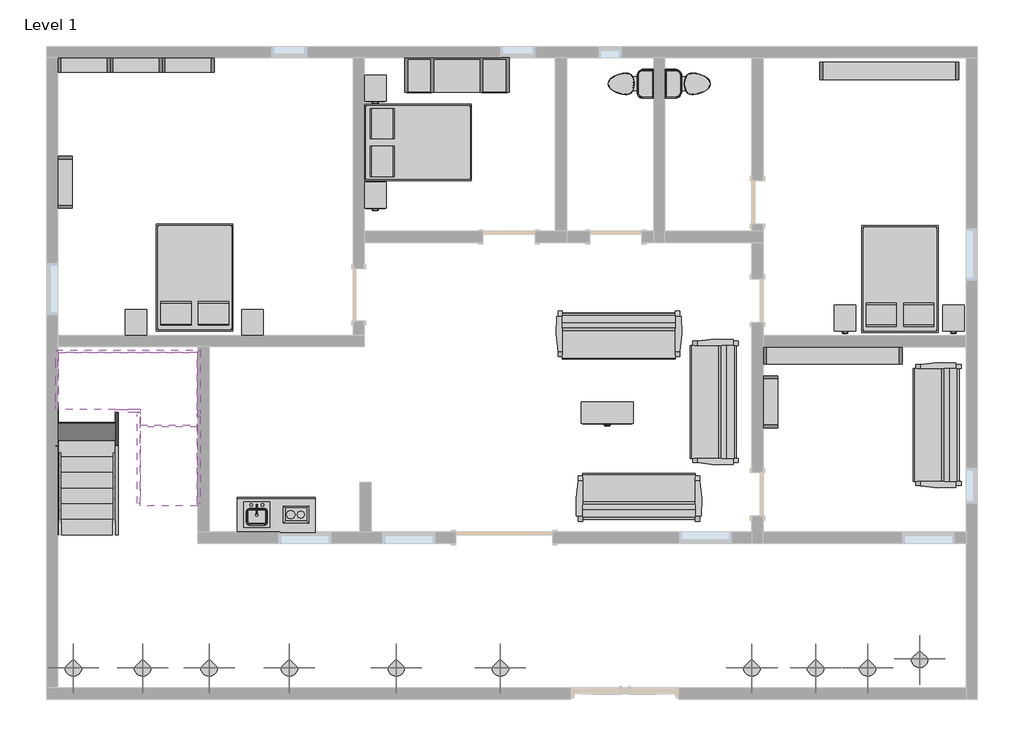
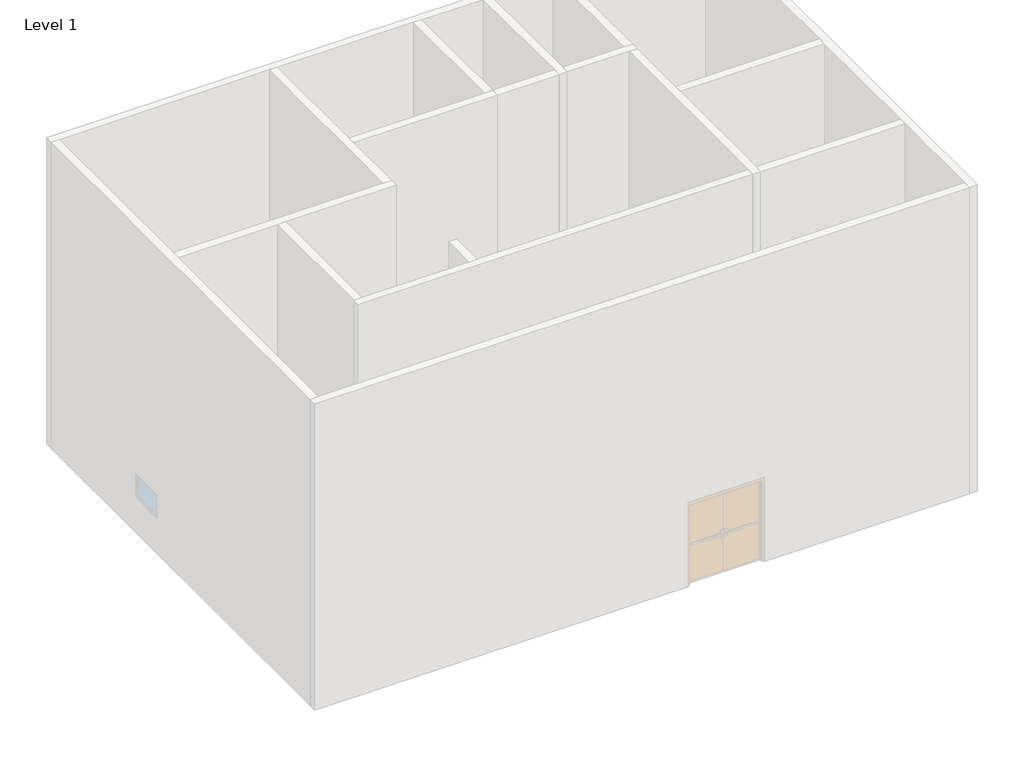
# One storey, part 4 of 4: 23 furniture elements, 10 geographic elements, 8 members, 3 flow terminals, 2 proxies, 2 stair flights, 1 slab.
"""IFC4 building model written with IfcOpenShell, lengths in millimetres."""

from ifc_helpers import new_model, si_unit, frame, origin, place, context, project, spatial, polyline, outline, extrude, faceted_brep, transform, mapped, element, save
from components import m_cook_top_2_unit_305_x_457mm_ebea1746, m_kitchenette_small_1372mm_f81b7602, m_sink_kitchen_island_450_x_450mm_f969cf2d, m_toilet_domestic_3d_m_toilet_domestic_3d_5cb52bd4, m_toilet_domestic_3d_m_toilet_domestic_3d_183bbd19, m_bed_box_1346_x_1880mm_double_b32eb57e, m_cabinet_file_2_drawer_0380_x_0457mm_9eec7cff, m_cabinet_file_2_drawer_0915_x_0380mm_lat_9df0d5dd, m_counter_top_w_sink_hole_600mm_depth_edbb3572, m_entertainment_center_1830_x_1830_x_0610mm_f77a9b93, m_shelving_0915_x_0254_x_1830mm_1d5e155e, m_shelving_2440_x_0305_x_2134mm_59c1a9e4, m_sofa_pensi_2134mm_91f3548c, m_rpc_plant_tropical_agave_0_45_meters_eb57889b, non_monolithic_landing_ea8e6b74, stair_flight_50mm_tread_25mm_nosing_13mm_riser_f1e983ca, stair_flight_50mm_tread_25mm_nosing_13mm_riser_46b24cc8

model = new_model("IFC4")

# Units and contexts
model_context = context("Model", 3, world=origin())
ifc_project = project(units=[si_unit("LENGTHUNIT", "METRE", prefix="MILLI")], contexts=[model_context])

# Site, building, storey
site = spatial("IfcSite", under=ifc_project)
building = spatial("IfcBuilding", under=site)
storey = spatial("IfcBuildingStorey", under=building, Name="Level 1", Elevation=0.0)

# Proxies
placement = place(None, origin())
m_cook_top_2_unit_305_x_457mm_shape = m_cook_top_2_unit_305_x_457mm_ebea1746(model_context)
element("IfcBuildingElementProxy", 1, Name="M_Cook Top-2 Unit : 305 x 457mm", ObjectType="M_Cook Top-2 Unit : 305 x 457mm", at=placement, inside=storey, context=model_context, shape_type="MappedRepresentation", body=[
    mapped(m_cook_top_2_unit_305_x_457mm_shape, transform((-7821.7428819, 1103.8280728, 40.0), x_axis=(0.0, 1.0, 0.0), y_axis=(-1.0, 0.0, 0.0), z_axis=(0.0, 0.0, 1.0))),
])
m_kitchenette_small_1372mm_shape = m_kitchenette_small_1372mm_f81b7602(model_context)
element("IfcBuildingElementProxy", 2, Name="M_Kitchenette - Small : 1372mm", ObjectType="M_Kitchenette - Small : 1372mm", at=placement, inside=storey, context=model_context, shape_type="MappedRepresentation", body=[
    mapped(m_kitchenette_small_1372mm_shape, transform((-8213.7053824, 1485.0280728, 0.0), x_axis=(1.0, 0.0, 0.0), y_axis=(0.0, 1.0, 0.0), z_axis=(0.0, 0.0, 1.0))),
])

# Flow terminals
m_sink_kitchen_island_450_x_450mm_shape = m_sink_kitchen_island_450_x_450mm_f969cf2d(model_context)
element("IfcFlowTerminal", 3, ObjectType="M_Sink Kitchen-Island : 450 x 450mm", at=placement, inside=storey, context=model_context, shape_type="MappedRepresentation", body=[
    mapped(m_sink_kitchen_island_450_x_450mm_shape, transform((-8553.6569181, 1177.6826717, 40.0), x_axis=(1.0, 0.0, 0.0), y_axis=(0.0, 1.0, 0.0), z_axis=(0.0, 0.0, 1.0))),
])
m_toilet_domestic_3d_m_toilet_domestic_3d_shape = m_toilet_domestic_3d_m_toilet_domestic_3d_5cb52bd4(model_context)
m_toilet_domestic_3d_m_toilet_domestic_3d_2_shape = m_toilet_domestic_3d_m_toilet_domestic_3d_183bbd19(model_context)
element("IfcFlowTerminal", 4, ObjectType="M_Toilet-Domestic-3D : M_Toilet-Domestic-3D", at=placement, inside=storey, context=model_context, shape_type="MappedRepresentation", body=[
    mapped(m_toilet_domestic_3d_m_toilet_domestic_3d_shape, transform((-2061.6637048, 8753.2241001, 0.0), x_axis=(0.0, -1.0000000000000002, 0.0), y_axis=(1.0000000000000002, 0.0, 0.0), z_axis=(0.0, 0.0, 1.0))),
    mapped(m_toilet_domestic_3d_m_toilet_domestic_3d_2_shape, transform((-2061.6637048, 8753.2241001, 0.0), x_axis=(0.0, -1.0000000000000002, 0.0), y_axis=(1.0000000000000002, 0.0, 0.0), z_axis=(0.0, 0.0, 1.0))),
])
element("IfcFlowTerminal", 5, ObjectType="M_Toilet-Domestic-3D : M_Toilet-Domestic-3D", at=placement, inside=storey, context=model_context, shape_type="MappedRepresentation", body=[
    mapped(m_toilet_domestic_3d_m_toilet_domestic_3d_shape, transform((-872.2716501, 8753.2241001, 0.0), x_axis=(0.0, 1.0000000000000002, 0.0), y_axis=(-1.0000000000000002, 0.0, 0.0), z_axis=(0.0, 0.0, 1.0))),
    mapped(m_toilet_domestic_3d_m_toilet_domestic_3d_2_shape, transform((-872.2716501, 8753.2241001, 0.0), x_axis=(0.0, 1.0000000000000002, 0.0), y_axis=(-1.0000000000000002, 0.0, 0.0), z_axis=(0.0, 0.0, 1.0))),
])

# Furniture
m_bed_box_1346_x_1880mm_double_shape = m_bed_box_1346_x_1880mm_double_b32eb57e(model_context)
element("IfcFurniture", 6, ObjectType="M_Bed-Box : 1346 x 1880mm - Double", at=placement, inside=storey, context=model_context, shape_type="MappedRepresentation", body=[
    mapped(m_bed_box_1346_x_1880mm_double_shape, transform((-9290.8152185, 5112.7985646, 0.0), x_axis=(-1.0, 0.0, 0.0), y_axis=(0.0, -1.0, 0.0), z_axis=(0.0, 0.0, 1.0))),
])
element("IfcFurniture", 7, ObjectType="M_Bed-Box : 1346 x 1880mm - Double", at=placement, inside=storey, context=model_context, shape_type="MappedRepresentation", body=[
    mapped(m_bed_box_1346_x_1880mm_double_shape, transform((-5941.3971857, 7382.8756138, 0.0), x_axis=(0.0, 1.0, 0.0), y_axis=(-1.0, 0.0, 0.0), z_axis=(0.0, 0.0, 1.0))),
])
element("IfcFurniture", 8, ObjectType="M_Bed-Box : 1346 x 1880mm - Double", at=placement, inside=storey, context=model_context, shape_type="MappedRepresentation", body=[
    mapped(m_bed_box_1346_x_1880mm_double_shape, transform((3101.1847815, 5087.3985646, 0.0), x_axis=(-1.0000000000000004, 0.0, 0.0), y_axis=(0.0, -1.0000000000000004, 0.0), z_axis=(0.0, 0.0, 1.0))),
])
m_cabinet_file_2_drawer_0380_x_0457mm_shape = m_cabinet_file_2_drawer_0380_x_0457mm_9eec7cff(model_context)
element("IfcFurniture", 9, ObjectType="M_Cabinet-File 2 Drawer : 0380 x 0457mm", at=placement, inside=storey, context=model_context, shape_type="MappedRepresentation", body=[
    mapped(m_cabinet_file_2_drawer_0380_x_0457mm_shape, transform((-8485.4712305, 4701.6623729, 0.0), x_axis=(1.0, 0.0, 0.0), y_axis=(0.0, 1.0, 0.0), z_axis=(0.0, 0.0, 1.0))),
])
element("IfcFurniture", 10, ObjectType="M_Cabinet-File 2 Drawer : 0380 x 0457mm", at=placement, inside=storey, context=model_context, shape_type="MappedRepresentation", body=[
    mapped(m_cabinet_file_2_drawer_0380_x_0457mm_shape, transform((-10531.3712305, 4701.6623729, 0.0), x_axis=(1.0, 0.0, 0.0), y_axis=(0.0, 1.0, 0.0), z_axis=(0.0, 0.0, 1.0))),
])
element("IfcFurniture", 11, ObjectType="M_Cabinet-File 2 Drawer : 0380 x 0457mm", at=placement, inside=storey, context=model_context, shape_type="MappedRepresentation", body=[
    mapped(m_cabinet_file_2_drawer_0380_x_0457mm_shape, transform((-6329.0712305, 8816.6623729, 0.0), x_axis=(1.0, 0.0, 0.0), y_axis=(0.0, 1.0, 0.0), z_axis=(0.0, 0.0, 1.0))),
])
element("IfcFurniture", 12, ObjectType="M_Cabinet-File 2 Drawer : 0380 x 0457mm", at=placement, inside=storey, context=model_context, shape_type="MappedRepresentation", body=[
    mapped(m_cabinet_file_2_drawer_0380_x_0457mm_shape, transform((-6329.0712305, 6937.0623729, 0.0), x_axis=(1.0, 0.0, 0.0), y_axis=(0.0, 1.0, 0.0), z_axis=(0.0, 0.0, 1.0))),
])
element("IfcFurniture", 13, ObjectType="M_Cabinet-File 2 Drawer : 0380 x 0457mm", at=placement, inside=storey, context=model_context, shape_type="MappedRepresentation", body=[
    mapped(m_cabinet_file_2_drawer_0380_x_0457mm_shape, transform((1925.3287695, 4780.4623729, 0.0), x_axis=(1.0, 0.0, 0.0), y_axis=(0.0, 1.0, 0.0), z_axis=(0.0, 0.0, 1.0))),
])
element("IfcFurniture", 14, ObjectType="M_Cabinet-File 2 Drawer : 0380 x 0457mm", at=placement, inside=storey, context=model_context, shape_type="MappedRepresentation", body=[
    mapped(m_cabinet_file_2_drawer_0380_x_0457mm_shape, transform((3829.1287695, 4780.4623729, 0.0), x_axis=(1.0, 0.0, 0.0), y_axis=(0.0, 1.0, 0.0), z_axis=(0.0, 0.0, 1.0))),
])
m_cabinet_file_2_drawer_0915_x_0380mm_lat_shape = m_cabinet_file_2_drawer_0915_x_0380mm_lat_9df0d5dd(model_context)
element("IfcFurniture", 15, ObjectType="M_Cabinet-File 2 Drawer : 0915 x 0380mm Lat.", at=placement, inside=storey, context=model_context, shape_type="MappedRepresentation", body=[
    mapped(m_cabinet_file_2_drawer_0915_x_0380mm_lat_shape, transform((-2253.4712305, 3114.7623729, 0.0), x_axis=(1.0, 0.0, 0.0), y_axis=(0.0, 1.0, 0.0), z_axis=(0.0, 0.0, 1.0))),
])
m_counter_top_w_sink_hole_600mm_depth_shape = m_counter_top_w_sink_hole_600mm_depth_edbb3572(model_context)
element("IfcFurniture", 16, ObjectType="M_Counter Top w Sink Hole : 600mm Depth", at=placement, inside=storey, context=model_context, shape_type="MappedRepresentation", body=[
    mapped(m_counter_top_w_sink_hole_600mm_depth_shape, transform((-7680.5053824, 1485.0280728, 40.0), x_axis=(1.0, 0.0, 0.0), y_axis=(0.0, 1.0, 0.0), z_axis=(0.0, 0.0, 1.0))),
])
m_entertainment_center_1830_x_1830_x_0610mm_shape = m_entertainment_center_1830_x_1830_x_0610mm_f77a9b93(model_context)
element("IfcFurniture", 17, ObjectType="M_Entertainment center : 1830 x 1830 x 0610mm", at=placement, inside=storey, context=model_context, shape_type="MappedRepresentation", body=[
    mapped(m_entertainment_center_1830_x_1830_x_0610mm_shape, transform((-5021.9676775, 9310.8280728, 0.0), x_axis=(1.0, 0.0, 0.0), y_axis=(0.0, 1.0, 0.0), z_axis=(0.0, 0.0, 1.0))),
])
m_shelving_0915_x_0254_x_1830mm_shape = m_shelving_0915_x_0254_x_1830mm_1d5e155e(model_context)
element("IfcFurniture", 18, ObjectType="M_Shelving : 0915 x 0254 x 1830mm", at=placement, inside=storey, context=model_context, shape_type="MappedRepresentation", body=[
    mapped(m_shelving_0915_x_0254_x_1830mm_shape, transform((-11574.2676775, 9387.2280728, 0.0), x_axis=(1.0, 0.0, 0.0), y_axis=(0.0, 1.0, 0.0), z_axis=(0.0, 0.0, 1.0))),
])
element("IfcFurniture", 19, ObjectType="M_Shelving : 0915 x 0254 x 1830mm", at=placement, inside=storey, context=model_context, shape_type="MappedRepresentation", body=[
    mapped(m_shelving_0915_x_0254_x_1830mm_shape, transform((-10659.2676775, 9387.2280728, 0.0), x_axis=(1.0, 0.0, 0.0), y_axis=(0.0, 1.0, 0.0), z_axis=(0.0, 0.0, 1.0))),
])
element("IfcFurniture", 20, ObjectType="M_Shelving : 0915 x 0254 x 1830mm", at=placement, inside=storey, context=model_context, shape_type="MappedRepresentation", body=[
    mapped(m_shelving_0915_x_0254_x_1830mm_shape, transform((-9744.2676775, 9387.2280728, 0.0), x_axis=(1.0, 0.0, 0.0), y_axis=(0.0, 1.0, 0.0), z_axis=(0.0, 0.0, 1.0))),
])
element("IfcFurniture", 21, ObjectType="M_Shelving : 0915 x 0254 x 1830mm", at=placement, inside=storey, context=model_context, shape_type="MappedRepresentation", body=[
    mapped(m_shelving_0915_x_0254_x_1830mm_shape, transform((-12209.5676775, 7023.1280728, 0.0), x_axis=(0.0, 1.0, 0.0), y_axis=(-1.0, 0.0, 0.0), z_axis=(0.0, 0.0, 1.0))),
])
element("IfcFurniture", 22, ObjectType="M_Shelving : 0915 x 0254 x 1830mm", at=placement, inside=storey, context=model_context, shape_type="MappedRepresentation", body=[
    mapped(m_shelving_0915_x_0254_x_1830mm_shape, transform((182.4323225, 3162.3280728, 0.0), x_axis=(0.0, 1.0000000000000002, 0.0), y_axis=(-1.0000000000000002, 0.0, 0.0), z_axis=(0.0, 0.0, 1.0))),
])
m_shelving_2440_x_0305_x_2134mm_shape = m_shelving_2440_x_0305_x_2134mm_59c1a9e4(model_context)
element("IfcFurniture", 23, ObjectType="M_Shelving : 2440 x 0305 x 2134mm", at=placement, inside=storey, context=model_context, shape_type="MappedRepresentation", body=[
    mapped(m_shelving_2440_x_0305_x_2134mm_shape, transform((2574.0323225, 9283.9280728, 0.0), x_axis=(1.0, 0.0, 0.0), y_axis=(0.0, 1.0, 0.0), z_axis=(0.0, 0.0, 1.0))),
])
element("IfcFurniture", 24, ObjectType="M_Shelving : 2440 x 0305 x 2134mm", at=placement, inside=storey, context=model_context, shape_type="MappedRepresentation", body=[
    mapped(m_shelving_2440_x_0305_x_2134mm_shape, transform((1580.2323225, 3673.7280728, 0.0), x_axis=(-1.0000000000000004, 0.0, 0.0), y_axis=(0.0, -1.0000000000000004, 0.0), z_axis=(0.0, 0.0, 1.0))),
])
m_sofa_pensi_2134mm_shape = m_sofa_pensi_2134mm_91f3548c(model_context)
element("IfcFurniture", 25, ObjectType="M_Sofa-Pensi : 2134mm", at=placement, inside=storey, context=model_context, shape_type="MappedRepresentation", body=[
    mapped(m_sofa_pensi_2134mm_shape, transform((3135.9224864, 3034.8343228, 0.0), x_axis=(0.0, -1.0000000000000002, 0.0), y_axis=(1.0000000000000002, 0.0, 0.0), z_axis=(0.0, 0.0, 1.0))),
])
element("IfcFurniture", 26, ObjectType="M_Sofa-Pensi : 2134mm", at=placement, inside=storey, context=model_context, shape_type="MappedRepresentation", body=[
    mapped(m_sofa_pensi_2134mm_shape, transform((-780.4775136, 3440.9343228, 0.0), x_axis=(0.0, -1.0000000000000002, 0.0), y_axis=(1.0000000000000002, 0.0, 0.0), z_axis=(0.0, 0.0, 1.0))),
])
element("IfcFurniture", 27, ObjectType="M_Sofa-Pensi : 2134mm", at=placement, inside=storey, context=model_context, shape_type="MappedRepresentation", body=[
    mapped(m_sofa_pensi_2134mm_shape, transform((-2456.7739275, 4053.9182367, 0.0), x_axis=(1.0, 0.0, 0.0), y_axis=(0.0, 1.0, 0.0), z_axis=(0.0, 0.0, 1.0))),
])
element("IfcFurniture", 28, ObjectType="M_Sofa-Pensi : 2134mm", at=placement, inside=storey, context=model_context, shape_type="MappedRepresentation", body=[
    mapped(m_sofa_pensi_2134mm_shape, transform((-1543.9614275, 1763.3379088, 0.0), x_axis=(-1.0, 0.0, 0.0), y_axis=(0.0, -1.0, 0.0), z_axis=(0.0, 0.0, 1.0))),
])

# Geographic elements
m_rpc_plant_tropical_agave_0_45_meters_shape = m_rpc_plant_tropical_agave_0_45_meters_eb57889b(model_context)
element("IfcGeographicElement", 29, ObjectType="M_RPC Plant - Tropical : Agave - 0.45 Meters", at=placement, inside=storey, context=model_context, shape_type="MappedRepresentation", body=[
    mapped(m_rpc_plant_tropical_agave_0_45_meters_shape, transform((-9376.1643486, -1510.9719272, 0.0), x_axis=(1.0, 0.0, 0.0), y_axis=(0.0, 1.0, 0.0), z_axis=(0.0, 0.0, 1.0))),
])
element("IfcGeographicElement", 30, ObjectType="M_RPC Plant - Tropical : Agave - 0.45 Meters", at=placement, inside=storey, context=model_context, shape_type="MappedRepresentation", body=[
    mapped(m_rpc_plant_tropical_agave_0_45_meters_shape, transform((-7966.3643486, -1510.9719272, 0.0), x_axis=(1.0, 0.0, 0.0), y_axis=(0.0, 1.0, 0.0), z_axis=(0.0, 0.0, 1.0))),
])
element("IfcGeographicElement", 31, ObjectType="M_RPC Plant - Tropical : Agave - 0.45 Meters", at=placement, inside=storey, context=model_context, shape_type="MappedRepresentation", body=[
    mapped(m_rpc_plant_tropical_agave_0_45_meters_shape, transform((-6088.3643486, -1510.9719272, 0.0), x_axis=(1.0, 0.0, 0.0), y_axis=(0.0, 1.0, 0.0), z_axis=(0.0, 0.0, 1.0))),
])
element("IfcGeographicElement", 32, ObjectType="M_RPC Plant - Tropical : Agave - 0.45 Meters", at=placement, inside=storey, context=model_context, shape_type="MappedRepresentation", body=[
    mapped(m_rpc_plant_tropical_agave_0_45_meters_shape, transform((-4259.5643486, -1510.9719272, 0.0), x_axis=(1.0, 0.0, 0.0), y_axis=(0.0, 1.0, 0.0), z_axis=(0.0, 0.0, 1.0))),
])
element("IfcGeographicElement", 33, ObjectType="M_RPC Plant - Tropical : Agave - 0.45 Meters", at=placement, inside=storey, context=model_context, shape_type="MappedRepresentation", body=[
    mapped(m_rpc_plant_tropical_agave_0_45_meters_shape, transform((160.0356514, -1510.9719272, 0.0), x_axis=(1.0, 0.0, 0.0), y_axis=(0.0, 1.0, 0.0), z_axis=(0.0, 0.0, 1.0))),
])
element("IfcGeographicElement", 34, ObjectType="M_RPC Plant - Tropical : Agave - 0.45 Meters", at=placement, inside=storey, context=model_context, shape_type="MappedRepresentation", body=[
    mapped(m_rpc_plant_tropical_agave_0_45_meters_shape, transform((1279.2356514, -1510.9719272, 0.0), x_axis=(1.0, 0.0, 0.0), y_axis=(0.0, 1.0, 0.0), z_axis=(0.0, 0.0, 1.0))),
])
element("IfcGeographicElement", 35, ObjectType="M_RPC Plant - Tropical : Agave - 0.45 Meters", at=placement, inside=storey, context=model_context, shape_type="MappedRepresentation", body=[
    mapped(m_rpc_plant_tropical_agave_0_45_meters_shape, transform((3108.0356514, -1358.5719272, 0.0), x_axis=(1.0, 0.0, 0.0), y_axis=(0.0, 1.0, 0.0), z_axis=(0.0, 0.0, 1.0))),
])
element("IfcGeographicElement", 36, ObjectType="M_RPC Plant - Tropical : Agave - 0.45 Meters", at=placement, inside=storey, context=model_context, shape_type="MappedRepresentation", body=[
    mapped(m_rpc_plant_tropical_agave_0_45_meters_shape, transform((2193.6356514, -1510.9719272, 0.0), x_axis=(1.0, 0.0, 0.0), y_axis=(0.0, 1.0, 0.0), z_axis=(0.0, 0.0, 1.0))),
])
element("IfcGeographicElement", 37, ObjectType="M_RPC Plant - Tropical : Agave - 0.45 Meters", at=placement, inside=storey, context=model_context, shape_type="MappedRepresentation", body=[
    mapped(m_rpc_plant_tropical_agave_0_45_meters_shape, transform((-11762.1643486, -1510.9719272, 0.0), x_axis=(1.0, 0.0, 0.0), y_axis=(0.0, 1.0, 0.0), z_axis=(0.0, 0.0, 1.0))),
])
element("IfcGeographicElement", 38, ObjectType="M_RPC Plant - Tropical : Agave - 0.45 Meters", at=placement, inside=storey, context=model_context, shape_type="MappedRepresentation", body=[
    mapped(m_rpc_plant_tropical_agave_0_45_meters_shape, transform((-10542.9643486, -1510.9719272, 0.0), x_axis=(1.0, 0.0, 0.0), y_axis=(0.0, 1.0, 0.0), z_axis=(0.0, 0.0, 1.0))),
])

# Members
element("IfcMember", 39, ObjectType="Stringer - 50mm Width", at=placement, inside=storey, context=model_context, shape_type="SweptSolid", body=[
    extrude(outline(polyline([(827.4280728, 0.0), (827.4280728, 215.089535), (3037.2590763, 1612.6111183), (3153.1281364, 1212.6111183), (1235.6868056, 0.0), (827.4280728, 0.0)])), frame((-12072.1805681, 0.0, 0.0), z_axis=(1.0, 0.0, 0.0), x_axis=(0.0, 1.0, 0.0)), (0.0, 0.0, 1.0), 50.0),
])
element("IfcMember", 40, ObjectType="Stringer - 50mm Width", at=placement, inside=storey, context=model_context, shape_type="SweptSolid", body=[
    extrude(outline(polyline([(827.4280728, 0.0), (827.4280728, 215.089535), (2977.4280728, 1574.7733295), (2977.4280728, 1101.4964536), (1235.6868056, 0.0), (827.4280728, 0.0)])), frame((-11022.1547869, 0.0, 0.0), z_axis=(1.0, 0.0, 0.0), x_axis=(0.0, 1.0, 0.0)), (0.0, 0.0, 1.0), 50.0),
])
element("IfcMember", 41, ObjectType="Stringer - 50mm Width", at=placement, inside=storey, context=model_context, shape_type="SweptSolid", body=[
    extrude(outline(polyline([(3017.5970692, 1612.6111183), (2901.7280092, 1212.6111183), (1377.4280728, 2176.5952678), (1377.4280728, 2649.8721437), (3017.5970692, 1612.6111183)])), frame((-9585.5547869, 0.0, 0.0), z_axis=(1.0, 0.0, 0.0), x_axis=(0.0, 1.0, 0.0)), (0.0, 0.0, 1.0), 50.0),
])
element("IfcMember", 42, ObjectType="Stringer - 50mm Width", at=placement, inside=storey, context=model_context, shape_type="SweptSolid", body=[
    extrude(outline(polyline([(2977.4280728, 1638.0144362), (2977.4280728, 1212.6111183), (2901.7280092, 1212.6111183), (1377.4280728, 2176.5952678), (1377.4280728, 2649.8721437), (2977.4280728, 1638.0144362)])), frame((-10635.5805681, 0.0, 0.0), z_axis=(1.0, 0.0, 0.0), x_axis=(0.0, 1.0, 0.0)), (0.0, 0.0, 1.0), 50.0),
])
element("IfcMember", 43, ObjectType="Stringer - 50mm Width", at=placement, inside=storey, context=model_context, shape_type="Brep", body=[
    faceted_brep([(-9585.5547869, 3017.5970692, 1612.6111183), (-9535.5547869, 3017.5970692, 1612.6111183), (-9535.5547869, 4077.453854, 1612.6111183), (-9585.5547869, 4027.453854, 1612.6111183), (-9585.5547869, 2901.7280092, 1212.6111183), (-9585.5547869, 4027.453854, 1212.6111183), (-9535.5547869, 2901.7280092, 1212.6111183), (-9535.5547869, 4077.453854, 1212.6111183)], [[[0, 1, 2, 3]], [[4, 0, 3, 5]], [[6, 4, 5, 7]], [[1, 6, 7, 2]], [[1, 0, 4, 6]], [[2, 7, 5, 3]]]),
])
element("IfcMember", 44, ObjectType="Stringer - 50mm Width", at=placement, inside=storey, context=model_context, shape_type="SweptSolid", body=[
    extrude(outline(polyline([(-9535.5547869, 4077.453854), (-9585.5547869, 4027.453854), (-12022.1805681, 4027.453854), (-12072.1805681, 4077.453854), (-9535.5547869, 4077.453854)])), frame((0.0, 0.0, 1212.6111183), z_axis=(0.0, 0.0, 1.0), x_axis=(1.0, 0.0, 0.0)), (0.0, 0.0, 1.0), 400.0),
])
element("IfcMember", 45, ObjectType="Stringer - 50mm Width", at=placement, inside=storey, context=model_context, shape_type="Brep", body=[
    faceted_brep([(-12022.1805681, 4027.453854, 1612.6111183), (-12072.1805681, 4077.453854, 1612.6111183), (-12072.1805681, 3037.2590763, 1612.6111183), (-12022.1805681, 3037.2590763, 1612.6111183), (-12022.1805681, 4027.453854, 1212.6111183), (-12022.1805681, 3153.1281364, 1212.6111183), (-12072.1805681, 4077.453854, 1212.6111183), (-12072.1805681, 3153.1281364, 1212.6111183)], [[[0, 1, 2, 3]], [[4, 0, 3, 5]], [[6, 4, 5, 7]], [[1, 6, 7, 2]], [[1, 0, 4, 6]], [[2, 7, 5, 3]]]),
])
element("IfcMember", 46, ObjectType="Stringer - 50mm Width", at=placement, inside=storey, context=model_context, shape_type="SweptSolid", body=[
    extrude(outline(polyline([(-11022.1547869, 2977.4280728), (-11022.1547869, 3027.4280728), (-10585.5805681, 3027.4280728), (-10585.5805681, 2977.4280728), (-11022.1547869, 2977.4280728)])), frame((0.0, 0.0, 1212.6111183), z_axis=(0.0, 0.0, 1.0), x_axis=(1.0, 0.0, 0.0)), (0.0, 0.0, 1.0), 400.0),
])

# Slab
non_monolithic_landing_shape = non_monolithic_landing_ea8e6b74(model_context)
element("IfcSlab", 47, ObjectType="Non-Monolithic Landing", at=placement, inside=storey, context=model_context, shape_type="MappedRepresentation", body=[
    mapped(non_monolithic_landing_shape, transform((0.0, 0.0, 0.0), x_axis=(1.0, 0.0, 0.0), y_axis=(0.0, 1.0, 0.0), z_axis=(0.0, 0.0, 1.0))),
])

# Stair flights
stair_flight_50mm_tread_25mm_nosing_13mm_riser_shape = stair_flight_50mm_tread_25mm_nosing_13mm_riser_f1e983ca(model_context)
element("IfcStairFlight", 48, ObjectType="50mm Tread 25mm Nosing 13mm Riser", at=placement, inside=storey, context=model_context, shape_type="MappedRepresentation", body=[
    mapped(stair_flight_50mm_tread_25mm_nosing_13mm_riser_shape, transform((0.0, 0.0, 0.0), x_axis=(1.0, 0.0, 0.0), y_axis=(0.0, 1.0, 0.0), z_axis=(0.0, 0.0, 1.0))),
])
stair_flight_50mm_tread_25mm_nosing_13mm_riser_2_shape = stair_flight_50mm_tread_25mm_nosing_13mm_riser_46b24cc8(model_context)
element("IfcStairFlight", 49, ObjectType="50mm Tread 25mm Nosing 13mm Riser", at=placement, inside=storey, context=model_context, shape_type="MappedRepresentation", body=[
    mapped(stair_flight_50mm_tread_25mm_nosing_13mm_riser_2_shape, transform((0.0, 0.0, 0.0), x_axis=(1.0, 0.0, 0.0), y_axis=(0.0, 1.0, 0.0), z_axis=(0.0, 0.0, 1.0))),
])

save(model, "model.ifc")

# Revit data of these elements
# Type "M_Cook Top-2 Unit : 305 x 457mm"
#   Counter Height = 900 mm
#   Depth = 457 mm
#   Width = 305 mm
#   Burner Material = Steel, Chrome Plated
#   Cooktop Material = Steel, Polished
#   Default Elevation = 0
# Type "M_Kitchenette - Small : 1372mm"
#   Width = 1372 mm
#   Height = 900 mm
#   Depth = 610 mm
#   Toe Depth = 35 mm
#   Toe Height = 100 mm
#   Cabinet Material = Cabinets
#   Door/Drawer Material = Cabinets
#   Handle Material = Cabinets - Handles
#   Default Elevation = 0
# Type "M_Sink Kitchen-Island : 450 x 450mm"
#   Counter Height [instance default] = 900 mm
#   Depth = 450 mm
#   Width = 450 mm
#   Fixture Material = Steel, Polished
#   Sink Material = Steel, Polished
#   Default Elevation = 0
# Type "M_Toilet-Domestic-3D : M_Toilet-Domestic-3D"
#   Bowl/Basin Material = Porcelain, Linen
#   Seat Material = Laminate, Linen, Matte
#   Default Elevation = 0
# Type "M_Bed-Box : 1346 x 1880mm - Double"
#   Length = 1880 mm
#   Width = 1346 mm
#   Frame Material = Birch
#   Mattress Material = Linen, White
#   Default Elevation = 0
# Type "M_Cabinet-File 2 Drawer : 0380 x 0457mm"
#   Depth = 457 mm
#   Height = 734 mm
#   Width = 380 mm
#   Cabinet Material = Steel, Paint Finish, Ivory, Glossy
#   Handle Material = Steel, Chrome Plated
#   Default Elevation = 0
# Type "M_Cabinet-File 2 Drawer : 0915 x 0380mm Lat."
#   Depth = 380 mm
#   Height = 711 mm
#   Width = 915 mm
#   Cabinet Material = Steel, Paint Finish, Ivory, Glossy
#   Handle Material = Steel, Chrome Plated
#   Default Elevation = 0
# Type "M_Counter Top w Sink Hole : 600mm Depth"
#   Counter Thickness = 40 mm
#   Depth = 625 mm
#   Height = 900 mm
#   Length [instance default] = 2500 mm
#   Sink Location [instance default] = 1200 mm
#   Sink Location To Wall [instance default] = 100 mm
#   Sink Opening Depth [instance default] = 378 mm
#   Sink Opening Width [instance default] = 587 mm
#   Counter Top Material = none
#   Default Elevation = 0
# Type "M_Entertainment center : 1830 x 1830 x 0610mm"
#   Center Width = 813 mm
#   Depth = 610 mm
#   Height = 1830 mm
#   Width = 1830 mm
#   Material = Laminate, Ivory, Matte
#   Default Elevation = 0
# Type "M_Shelving : 0915 x 0254 x 1830mm"
#   Depth = 254 mm
#   Height = 1830 mm
#   Width = 915 mm
#   Material = Birch
#   Default Elevation = 0
# Type "M_Shelving : 2440 x 0305 x 2134mm"
#   Depth = 305 mm
#   Height = 2134 mm
#   Width = 2440 mm
#   Material = Laminate, Ivory, Matte
#   Default Elevation = 0
# Type "M_Sofa-Pensi : 2134mm"
#   Length = 2134 mm
#   Sofa Material = Linen, Beige
#   Frame Material = Steel, Chrome Plated
#   Default Elevation = 0
# Type "M_RPC Plant - Tropical : Agave - 0.45 Meters"
#   built-in parameter 1005198 = "{2, 15},{39, RPC-16-G1GJ-63FX-7K5P-N000-ST1L-LVER-AU},{1, 0},{1, 0},{2, 13},{1, 8},{5, Color},{1, 0},{1, 0},{3, 0.8},{3, 0.8},{3, 0.8},{1, 8},{7, BBoxMin},{1, 0},{1, 0},{1, 0},{1, 0},{1, 0},{1, 8},{7, BBoxMax},{1, 0},{1, 0},{1, 0},{1, 0},{1, 0},{2, 11},{9, RPCTypeId},{1, 0},{1, 0},{39, RPC-16-G1GJ-63FX-7K5P-N000-ST1L-LVER-AU},{1, 6},{14, RPCPlantHeight},{1, 0},{1, 0},{7, 1.47638},{2, 11},{7, keyword},{1, 0},{1, 0},{35, :RPCs:Plants [General]:Geometry:RPC},{2, 11},{8, category},{1, 0},{1, 0},{16, Plants [General]},{2, 11},{12, LocalizedUID},{1, 0},{1, 0},{5, Agave},{2, 14},{6, Height},{1, 0},{1, 0},{7, 1.47638},{1, 2},{16, Cast Reflections},{1, 0},{1, 0},{1, 0},{1, 2},{12, Cast Shadows},{1, 0},{1, 0},{1, 1},{1, 2},{9, Lock View},{1, 0},{1, 0},{1, 0},{1, 4},{5, ViewC},{1, 0},{1, 0},{1, 0},{21, assetlibrary_base.fbx},{1, 5},"
#   built-in parameter 1005195 = "RPC-16-G1GJ-63FX-7K5P-N000-ST1L-LVER-AU"
#   Type Comments = "Agave"
#   Height = 450 mm
#   Description = (empty or 0)
#   Default Elevation = 0
# Element 1 (IfcBuildingElementProxy, "M_Cook Top-2 Unit : 305 x 457mm")
#   Phase Created = New Construction
#   Materials on its faces: "Steel, Chrome Plated", "Steel, Polished"
# Element 2 (IfcBuildingElementProxy, "M_Kitchenette - Small : 1372mm")
#   Phase Created = New Construction
#   Materials on its faces: "Cabinets", "Cabinets - Handles"
# Element 3 (IfcFlowTerminal, "M_Sink Kitchen-Island : 450 x 450mm")
#   Mark = "3"
#   Counter Height = 900 mm
#   Phase Created = New Construction
#   Materials on its faces: "Steel, Polished"
# Element 4 (IfcFlowTerminal, "M_Toilet-Domestic-3D : M_Toilet-Domestic-3D")
#   Mark = "1"
#   Phase Created = New Construction
#   Materials on its faces: "Porcelain, Linen", "Laminate, Linen, Matte"
# Element 5 (IfcFlowTerminal, "M_Toilet-Domestic-3D : M_Toilet-Domestic-3D")
#   Mark = "2"
#   Phase Created = New Construction
#   Materials on its faces: "Porcelain, Linen", "Laminate, Linen, Matte"
# Elements 6, 7, 8 (IfcFurniture, "M_Bed-Box : 1346 x 1880mm - Double")
#   Phase Created = New Construction
#   Materials on its faces: "Birch", "Linen, White"
# Elements 9, 10, 11, 12, 13, 14 (IfcFurniture, "M_Cabinet-File 2 Drawer : 0380 x 0457mm")
#   Phase Created = New Construction
#   Materials on its faces: "Steel, Chrome Plated", "Steel, Paint Finish, Ivory, Glossy"
# Element 15 (IfcFurniture, "M_Cabinet-File 2 Drawer : 0915 x 0380mm Lat.")
#   Phase Created = New Construction
#   Materials on its faces: "Steel, Chrome Plated", "Steel, Paint Finish, Ivory, Glossy"
# Element 16 (IfcFurniture, "M_Counter Top w Sink Hole : 600mm Depth")
#   Sink Opening Width = 400 mm
#   Sink Opening Depth = 350 mm
#   Sink Location To Wall = 165 mm
#   Sink Location = 350 mm
#   Length = 1372 mm
#   Phase Created = New Construction
#   Materials on its faces: "Counter Top"
# Element 17 (IfcFurniture, "M_Entertainment center : 1830 x 1830 x 0610mm")
#   Phase Created = New Construction
#   Materials on its faces: "Laminate, Ivory, Matte", "Steel, Chrome Plated", "Glass - Clear, Grey"
# Elements 18, 19, 20, 21, 22 (IfcFurniture, "M_Shelving : 0915 x 0254 x 1830mm")
#   Phase Created = New Construction
#   Materials on its faces: "Birch"
# Elements 23, 24 (IfcFurniture, "M_Shelving : 2440 x 0305 x 2134mm")
#   Phase Created = New Construction
#   Materials on its faces: "Laminate, Ivory, Matte"
# Elements 25, 26, 27, 28 (IfcFurniture, "M_Sofa-Pensi : 2134mm")
#   Phase Created = New Construction
#   Materials on its faces: "Linen, Beige", "Steel, Chrome Plated"
# Elements 29, 30, 31, 32, 33, 34, 35, 36, 37, 38 (IfcGeographicElement, "M_RPC Plant - Tropical : Agave - 0.45 Meters")
#   Phase Created = New Construction
# Elements 39, 40, 41, 42, 43, 44, 45, 46 (IfcMember, "Stringer - 50mm Width")
#   Phase Created = New Construction
# Element 47 (IfcSlab, "Non-Monolithic Landing")
#   Phase Created = New Construction
# Elements 48, 49 (IfcStairFlight, "50mm Tread 25mm Nosing 13mm Riser")
#   Phase Created = New Construction
# Materials
#   "Steel, Chrome Plated": class "Metal", colour RGB 244 244 244, transparency 0, Description = "Chromiuim plated steel", Cost = 0
#   "Steel, Polished": class "Metal", colour RGB 57 57 57, transparency 0, Description = "Polished steel", Cost = 0
#   "Cabinets": colour RGB 249 249 249, transparency 0
#   "Cabinets - Handles": class "Metal", colour RGB 57 57 57, transparency 0
#   "Porcelain, Linen": class "Ceramic", colour RGB 249 239 230, transparency 0, Description = "Porcelain, linen", Cost = 0
#   "Laminate, Linen, Matte": class "Plastic", colour RGB 249 239 230, transparency 0, Description = "Plastic Laminate - Linen, Matte", Cost = 0
#   "Birch": class "Wood", colour RGB 224 178 126, transparency 0, Description = "Betula Alleghaniensis", Cost = 0
#   "Linen, White": class "Textile", colour RGB 247 247 239, transparency 0, Description = "Linen, white", Cost = 0
#   "Steel, Paint Finish, Ivory, Glossy": class "Metal", colour RGB 247 247 239, transparency 0, Description = "Steel, paint finish, ivory, glossy", Cost = 0
#   "Laminate, Ivory, Matte": class "Plastic", colour RGB 247 247 229, transparency 0, Description = "Plastic Laminate - Ivory, Matte", Cost = 0
#   "Linen, Beige": class "Textile", colour RGB 249 239 230, transparency 0, Description = "Linen, beige", Cost = 0
#   "Counter Top": class "Wood", colour RGB 226 177 128, transparency 0
#   "Glass - Clear, Grey": class "Glass", colour RGB 252 255 255, transparency 0.64
